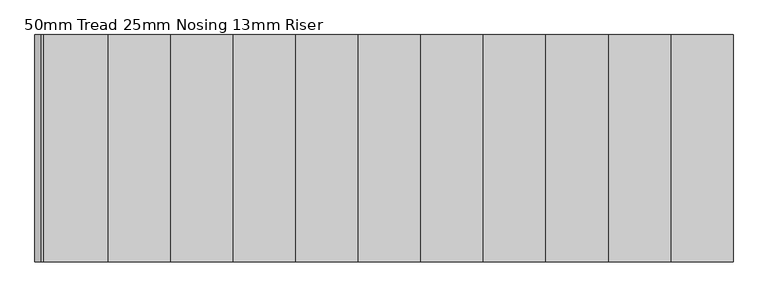
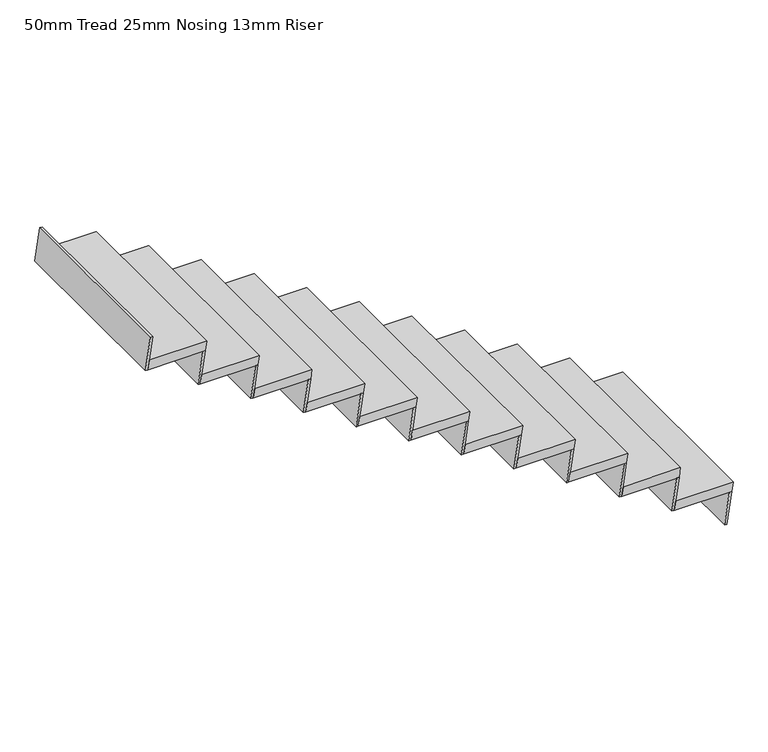
"""IFC4 building model written with IfcOpenShell, lengths in millimetres: stair flight geometry, 50mm Tread 25mm Nosing 13mm Riser."""

from ifc_helpers import new_model, si_unit, frame, origin, place, context, project, spatial, polyline, outline, extrude, source, transform, mapped, element, save


def stair_flight_50mm_tread_25mm_nosing_13mm_riser_1450225a(model_context):
    return source(origin(), model_context, "Body", "SweptSolid", [
        extrude(outline(polyline([(1043.4782609, -2691.9701746), (1043.4782609, -2991.9701746), (993.4782609, -2999.1576746), (993.4782609, -2699.1576746), (1043.4782609, -2691.9701746)])), frame((0.0, -3816.2148449, 0.0), z_axis=(0.0, 1.0, 0.0), x_axis=(0.0, 0.0, 1.0)), (0.0, 0.0, 1.0), 1000.0257813),
        extrude(outline(polyline([(993.4782609, -2699.1576746), (993.4782609, -2711.7861646), (819.5652174, -2736.7861646), (819.5652174, -2724.1576746), (993.4782609, -2699.1576746)])), frame((0.0, -3816.2148449, 0.0), z_axis=(0.0, 1.0, 0.0), x_axis=(0.0, 0.0, 1.0)), (0.0, 0.0, 1.0), 1000.0257813),
        extrude(outline(polyline([(1167.3913043, -2974.1576746), (1167.3913043, -2986.7861646), (993.4782609, -3011.7861646), (993.4782609, -2999.1576746), (1167.3913043, -2974.1576746)])), frame((0.0, -3816.2148449, 0.0), z_axis=(0.0, 1.0, 0.0), x_axis=(0.0, 0.0, 1.0)), (0.0, 0.0, 1.0), 1000.0257813),
        extrude(outline(polyline([(1217.3913043, -2966.9701746), (1217.3913043, -3266.9701746), (1167.3913043, -3274.1576746), (1167.3913043, -2974.1576746), (1217.3913043, -2966.9701746)])), frame((0.0, -3816.2148449, 0.0), z_axis=(0.0, 1.0, 0.0), x_axis=(0.0, 0.0, 1.0)), (0.0, 0.0, 1.0), 1000.0257813),
        extrude(outline(polyline([(1341.3043478, -3249.1576746), (1341.3043478, -3261.7861646), (1167.3913043, -3286.7861646), (1167.3913043, -3274.1576746), (1341.3043478, -3249.1576746)])), frame((0.0, -3816.2148449, 0.0), z_axis=(0.0, 1.0, 0.0), x_axis=(0.0, 0.0, 1.0)), (0.0, 0.0, 1.0), 1000.0257813),
        extrude(outline(polyline([(1391.3043478, -3241.9701746), (1391.3043478, -3541.9701746), (1341.3043478, -3549.1576746), (1341.3043478, -3249.1576746), (1391.3043478, -3241.9701746)])), frame((0.0, -3816.2148449, 0.0), z_axis=(0.0, 1.0, 0.0), x_axis=(0.0, 0.0, 1.0)), (0.0, 0.0, 1.0), 1000.0257813),
        extrude(outline(polyline([(1515.2173913, -3524.1576746), (1515.2173913, -3536.7861646), (1341.3043478, -3561.7861646), (1341.3043478, -3549.1576746), (1515.2173913, -3524.1576746)])), frame((0.0, -3816.2148449, 0.0), z_axis=(0.0, 1.0, 0.0), x_axis=(0.0, 0.0, 1.0)), (0.0, 0.0, 1.0), 1000.0257813),
        extrude(outline(polyline([(1565.2173913, -3516.9701746), (1565.2173913, -3816.9701746), (1515.2173913, -3824.1576746), (1515.2173913, -3524.1576746), (1565.2173913, -3516.9701746)])), frame((0.0, -3816.2148449, 0.0), z_axis=(0.0, 1.0, 0.0), x_axis=(0.0, 0.0, 1.0)), (0.0, 0.0, 1.0), 1000.0257813),
        extrude(outline(polyline([(1689.1304348, -3799.1576746), (1689.1304348, -3811.7861646), (1515.2173913, -3836.7861646), (1515.2173913, -3824.1576746), (1689.1304348, -3799.1576746)])), frame((0.0, -3816.2148449, 0.0), z_axis=(0.0, 1.0, 0.0), x_axis=(0.0, 0.0, 1.0)), (0.0, 0.0, 1.0), 1000.0257813),
        extrude(outline(polyline([(1739.1304348, -3791.9701746), (1739.1304348, -4091.9701746), (1689.1304348, -4099.1576746), (1689.1304348, -3799.1576746), (1739.1304348, -3791.9701746)])), frame((0.0, -3816.2148449, 0.0), z_axis=(0.0, 1.0, 0.0), x_axis=(0.0, 0.0, 1.0)), (0.0, 0.0, 1.0), 1000.0257813),
        extrude(outline(polyline([(1863.0434783, -4074.1576746), (1863.0434783, -4086.7861646), (1689.1304348, -4111.7861646), (1689.1304348, -4099.1576746), (1863.0434783, -4074.1576746)])), frame((0.0, -3816.2148449, 0.0), z_axis=(0.0, 1.0, 0.0), x_axis=(0.0, 0.0, 1.0)), (0.0, 0.0, 1.0), 1000.0257813),
        extrude(outline(polyline([(1913.0434783, -4066.9701746), (1913.0434783, -4366.9701746), (1863.0434783, -4374.1576746), (1863.0434783, -4074.1576746), (1913.0434783, -4066.9701746)])), frame((0.0, -3816.2148449, 0.0), z_axis=(0.0, 1.0, 0.0), x_axis=(0.0, 0.0, 1.0)), (0.0, 0.0, 1.0), 1000.0257813),
        extrude(outline(polyline([(2036.9565217, -4349.1576746), (2036.9565217, -4361.7861646), (1863.0434783, -4386.7861646), (1863.0434783, -4374.1576746), (2036.9565217, -4349.1576746)])), frame((0.0, -3816.2148449, 0.0), z_axis=(0.0, 1.0, 0.0), x_axis=(0.0, 0.0, 1.0)), (0.0, 0.0, 1.0), 1000.0257813),
        extrude(outline(polyline([(2086.9565217, -4341.9701746), (2086.9565217, -4641.9701746), (2036.9565217, -4649.1576746), (2036.9565217, -4349.1576746), (2086.9565217, -4341.9701746)])), frame((0.0, -3816.2148449, 0.0), z_axis=(0.0, 1.0, 0.0), x_axis=(0.0, 0.0, 1.0)), (0.0, 0.0, 1.0), 1000.0257813),
        extrude(outline(polyline([(2210.8695652, -4624.1576746), (2210.8695652, -4636.7861646), (2036.9565217, -4661.7861646), (2036.9565217, -4649.1576746), (2210.8695652, -4624.1576746)])), frame((0.0, -3816.2148449, 0.0), z_axis=(0.0, 1.0, 0.0), x_axis=(0.0, 0.0, 1.0)), (0.0, 0.0, 1.0), 1000.0257813),
        extrude(outline(polyline([(2260.8695652, -4616.9701746), (2260.8695652, -4916.9701746), (2210.8695652, -4924.1576746), (2210.8695652, -4624.1576746), (2260.8695652, -4616.9701746)])), frame((0.0, -3816.2148449, 0.0), z_axis=(0.0, 1.0, 0.0), x_axis=(0.0, 0.0, 1.0)), (0.0, 0.0, 1.0), 1000.0257813),
        extrude(outline(polyline([(2384.7826087, -4899.1576746), (2384.7826087, -4911.7861646), (2210.8695652, -4936.7861646), (2210.8695652, -4924.1576746), (2384.7826087, -4899.1576746)])), frame((0.0, -3816.2148449, 0.0), z_axis=(0.0, 1.0, 0.0), x_axis=(0.0, 0.0, 1.0)), (0.0, 0.0, 1.0), 1000.0257813),
        extrude(outline(polyline([(2434.7826087, -4891.9701746), (2434.7826087, -5191.9701746), (2384.7826087, -5199.1576746), (2384.7826087, -4899.1576746), (2434.7826087, -4891.9701746)])), frame((0.0, -3816.2148449, 0.0), z_axis=(0.0, 1.0, 0.0), x_axis=(0.0, 0.0, 1.0)), (0.0, 0.0, 1.0), 1000.0257813),
        extrude(outline(polyline([(2558.6956522, -5174.1576746), (2558.6956522, -5186.7861646), (2384.7826087, -5211.7861646), (2384.7826087, -5199.1576746), (2558.6956522, -5174.1576746)])), frame((0.0, -3816.2148449, 0.0), z_axis=(0.0, 1.0, 0.0), x_axis=(0.0, 0.0, 1.0)), (0.0, 0.0, 1.0), 1000.0257813),
        extrude(outline(polyline([(2608.6956522, -5166.9701746), (2608.6956522, -5466.9701746), (2558.6956522, -5474.1576746), (2558.6956522, -5174.1576746), (2608.6956522, -5166.9701746)])), frame((0.0, -3816.2148449, 0.0), z_axis=(0.0, 1.0, 0.0), x_axis=(0.0, 0.0, 1.0)), (0.0, 0.0, 1.0), 1000.0257813),
        extrude(outline(polyline([(2732.6086957, -5449.1576746), (2732.6086957, -5461.7861646), (2558.6956522, -5486.7861646), (2558.6956522, -5474.1576746), (2732.6086957, -5449.1576746)])), frame((0.0, -3816.2148449, 0.0), z_axis=(0.0, 1.0, 0.0), x_axis=(0.0, 0.0, 1.0)), (0.0, 0.0, 1.0), 1000.0257813),
        extrude(outline(polyline([(2906.5217391, -5724.1576746), (2906.5217391, -5736.7861646), (2732.6086957, -5761.7861646), (2732.6086957, -5749.1576746), (2906.5217391, -5724.1576746)])), frame((0.0, -3816.2148449, 0.0), z_axis=(0.0, 1.0, 0.0), x_axis=(0.0, 0.0, 1.0)), (0.0, 0.0, 1.0), 1000.0257813),
        extrude(outline(polyline([(2782.6086957, -5441.9701746), (2782.6086957, -5741.9701746), (2732.6086957, -5749.1576746), (2732.6086957, -5449.1576746), (2782.6086957, -5441.9701746)])), frame((0.0, -3816.2148449, 0.0), z_axis=(0.0, 1.0, 0.0), x_axis=(0.0, 0.0, 1.0)), (0.0, 0.0, 1.0), 1000.0257813),
    ])


if __name__ == "__main__":
    model = new_model("IFC4")
    model_context = context("Model", 3, world=origin())
    ifc_project = project(units=[si_unit("LENGTHUNIT", "METRE", prefix="MILLI")], contexts=[model_context])
    site = spatial("IfcSite", under=ifc_project)
    building = spatial("IfcBuilding", under=site)
    placement = place(None, origin())
    stair_flight_50mm_tread_25mm_nosing_13mm_riser_shape = stair_flight_50mm_tread_25mm_nosing_13mm_riser_1450225a(model_context)
    element("IfcStairFlight", 1, ObjectType="50mm Tread 25mm Nosing 13mm Riser", at=placement, inside=building, context=model_context, shape_type="MappedRepresentation", body=[
        mapped(stair_flight_50mm_tread_25mm_nosing_13mm_riser_shape, transform((0.0, 0.0, 0.0), x_axis=(1.0, 0.0, 0.0), y_axis=(0.0, 1.0, 0.0), z_axis=(0.0, 0.0, 1.0))),
    ])
    save(model, "model.ifc")
